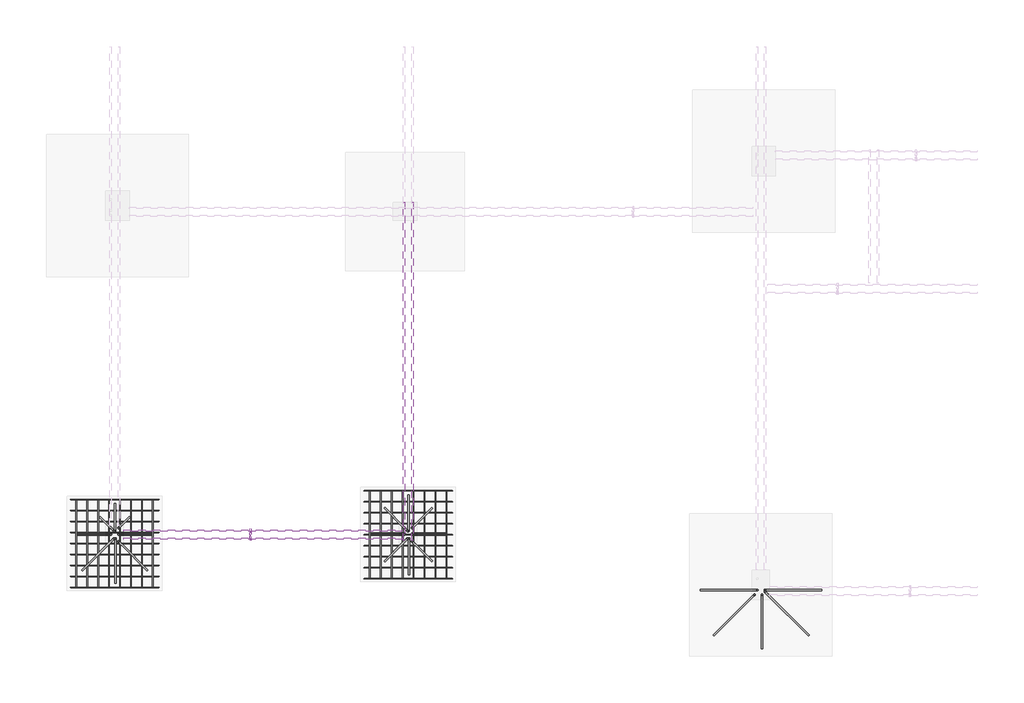
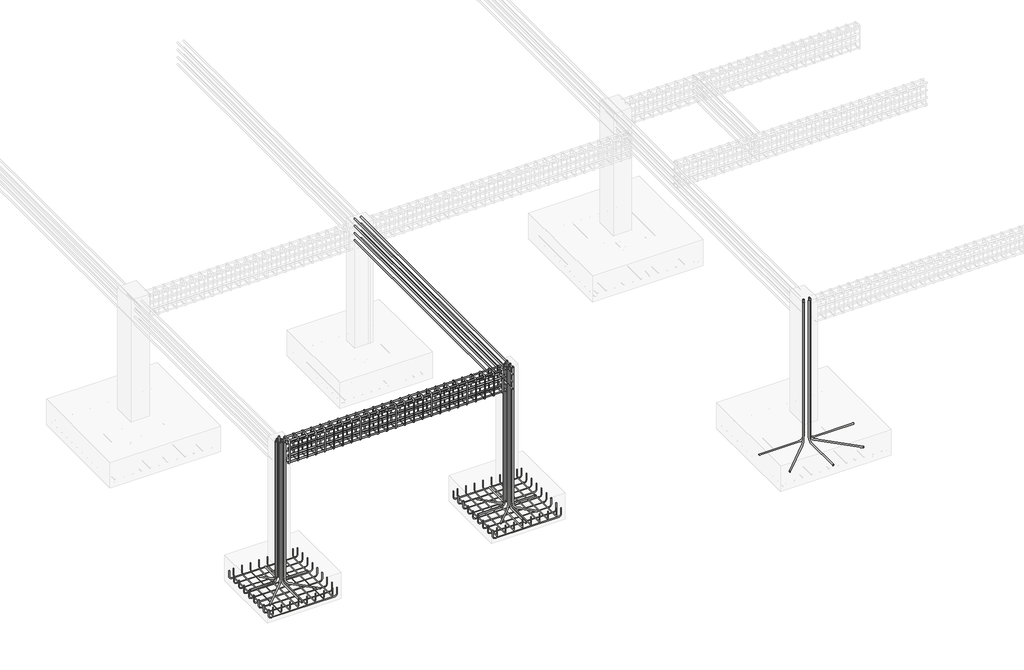
# One storey, part 2 of 10: 34 reinforcing bars.
"""IFC4 building model written with IfcOpenShell, lengths in millimetres."""

from ifc_helpers import new_model, si_unit, point, frame, origin, place, context, project, spatial, polyline, circle_curve, trimmed, segment, composite_curve, source, transform, mapped, element, save
from ifc_brep_helpers import swept_disk

model = new_model("IFC4")

# Units and contexts
model_context = context("Model", 3, world=origin())
ifc_project = project(units=[si_unit("LENGTHUNIT", "METRE", prefix="MILLI")], contexts=[model_context])

# Site, building, storey
site = spatial("IfcSite", under=ifc_project)
building = spatial("IfcBuilding", under=site)
storey = spatial("IfcBuildingStorey", under=building, Elevation=-2133.6)

# Reinforcing bars
placement = place(None, origin())
reinforcing_bar_shape = source(origin(), model_context, "Body", "SolidModel", [
    swept_disk(composite_curve([segment(polyline([(-4370.4164362, -2867.2780823, -2393.6), (-4370.4164362, -2867.2780823, -2504.1)]), True, "CONTINUOUS"), segment(trimmed(circle_curve(frame((-4405.1664362, -2867.2780823, -2504.1), z_axis=(0.0, 1.0, 0.0), x_axis=(34.75, 0.0, 0.0)), 34.75), [point((-4370.4164362, -2867.2780823, -2504.1))], [point((-4405.1664362, -2867.2780823, -2538.85))], True, "CARTESIAN"), True, "CONTINUOUS"), segment(polyline([(-4405.1664362, -2867.2780823, -2538.85), (-5465.3664362, -2867.2780823, -2538.85)]), True, "CONTINUOUS"), segment(trimmed(circle_curve(frame((-5465.3664362, -2867.2780823, -2504.1), z_axis=(0.0, 1.0, 0.0), x_axis=(0.0, 0.0, -34.75)), 34.75), [point((-5465.3664362, -2867.2780823, -2538.85))], [point((-5500.1164362, -2867.2780823, -2504.1))], True, "CARTESIAN"), True, "CONTINUOUS"), segment(polyline([(-5500.1164362, -2867.2780823, -2504.1), (-5500.1164362, -2867.2780823, -2393.6)]), True, "CONTINUOUS")], self_intersect=False), 4.75),
])
element("IfcReinforcingBar", 1, at=placement, inside=storey, context=model_context, shape_type="MappedRepresentation", body=[
    mapped(reinforcing_bar_shape, transform((0.0, 0.0, 0.0), x_axis=(1.0, 0.0, 0.0), y_axis=(0.0, 1.0, 0.0), z_axis=(0.0, 0.0, 1.0))),
    mapped(reinforcing_bar_shape, transform((0.0, -141.2125, 0.0), x_axis=(1.0, 0.0, 0.0), y_axis=(0.0, 1.0, 0.0), z_axis=(0.0, 0.0, 1.0))),
    mapped(reinforcing_bar_shape, transform((0.0, -282.425, 0.0), x_axis=(1.0, 0.0, 0.0), y_axis=(0.0, 1.0, 0.0), z_axis=(0.0, 0.0, 1.0))),
    mapped(reinforcing_bar_shape, transform((0.0, -423.6375, 0.0), x_axis=(1.0, 0.0, 0.0), y_axis=(0.0, 1.0, 0.0), z_axis=(0.0, 0.0, 1.0))),
    mapped(reinforcing_bar_shape, transform((0.0, -564.85, 0.0), x_axis=(1.0, 0.0, 0.0), y_axis=(0.0, 1.0, 0.0), z_axis=(0.0, 0.0, 1.0))),
    mapped(reinforcing_bar_shape, transform((0.0, -706.0625, 0.0), x_axis=(1.0, 0.0, 0.0), y_axis=(0.0, 1.0, 0.0), z_axis=(0.0, 0.0, 1.0))),
    mapped(reinforcing_bar_shape, transform((0.0, -847.275, 0.0), x_axis=(1.0, 0.0, 0.0), y_axis=(0.0, 1.0, 0.0), z_axis=(0.0, 0.0, 1.0))),
    mapped(reinforcing_bar_shape, transform((0.0, -988.4875, 0.0), x_axis=(1.0, 0.0, 0.0), y_axis=(0.0, 1.0, 0.0), z_axis=(0.0, 0.0, 1.0))),
    mapped(reinforcing_bar_shape, transform((0.0, -1129.7, 0.0), x_axis=(1.0, 0.0, 0.0), y_axis=(0.0, 1.0, 0.0), z_axis=(0.0, 0.0, 1.0))),
])
reinforcing_bar_2_shape = source(origin(), model_context, "Body", "SolidModel", [
    swept_disk(composite_curve([segment(polyline([(-4445.3743867, -3996.9780823, -2379.223371), (-4445.3743867, -3996.9780823, -2489.723371)]), True, "CONTINUOUS"), segment(trimmed(circle_curve(frame((-4445.3743867, -3962.2280823, -2489.723371), z_axis=(1.0, 0.0, 0.0), x_axis=(0.0, -34.75, 0.0)), 34.75), [point((-4445.3743867, -3996.9780823, -2489.723371))], [point((-4445.3743867, -3962.2280823, -2524.473371))], True, "CARTESIAN"), True, "CONTINUOUS"), segment(polyline([(-4445.3743867, -3962.2280823, -2524.473371), (-4445.3743867, -2902.0280823, -2524.473371)]), True, "CONTINUOUS"), segment(trimmed(circle_curve(frame((-4445.3743867, -2902.0280823, -2489.723371), z_axis=(1.0, 0.0, 0.0), x_axis=(0.0, 0.0, -34.75)), 34.75), [point((-4445.3743867, -2902.0280823, -2524.473371))], [point((-4445.3743867, -2867.2780823, -2489.723371))], True, "CARTESIAN"), True, "CONTINUOUS"), segment(polyline([(-4445.3743867, -2867.2780823, -2489.723371), (-4445.3743867, -2867.2780823, -2379.223371)]), True, "CONTINUOUS")], self_intersect=False), 4.75),
])
element("IfcReinforcingBar", 2, at=placement, inside=storey, context=model_context, shape_type="MappedRepresentation", body=[
    mapped(reinforcing_bar_2_shape, transform((0.0, 0.0, 0.0), x_axis=(1.0, 0.0, 0.0), y_axis=(0.0, 1.0, 0.0), z_axis=(0.0, 0.0, 1.0))),
    mapped(reinforcing_bar_2_shape, transform((-140.5079612, 0.0, 0.0), x_axis=(1.0, 0.0, 0.0), y_axis=(0.0, 1.0, 0.0), z_axis=(0.0, 0.0, 1.0))),
    mapped(reinforcing_bar_2_shape, transform((-281.0159224, 0.0, 0.0), x_axis=(1.0, 0.0, 0.0), y_axis=(0.0, 1.0, 0.0), z_axis=(0.0, 0.0, 1.0))),
    mapped(reinforcing_bar_2_shape, transform((-421.5238836, 0.0, 0.0), x_axis=(1.0, 0.0, 0.0), y_axis=(0.0, 1.0, 0.0), z_axis=(0.0, 0.0, 1.0))),
    mapped(reinforcing_bar_2_shape, transform((-562.0318448, 0.0, 0.0), x_axis=(1.0, 0.0, 0.0), y_axis=(0.0, 1.0, 0.0), z_axis=(0.0, 0.0, 1.0))),
    mapped(reinforcing_bar_2_shape, transform((-702.539806, 0.0, 0.0), x_axis=(1.0, 0.0, 0.0), y_axis=(0.0, 1.0, 0.0), z_axis=(0.0, 0.0, 1.0))),
    mapped(reinforcing_bar_2_shape, transform((-843.0477672, 0.0, 0.0), x_axis=(1.0, 0.0, 0.0), y_axis=(0.0, 1.0, 0.0), z_axis=(0.0, 0.0, 1.0))),
    mapped(reinforcing_bar_2_shape, transform((-983.5557284, 0.0, 0.0), x_axis=(1.0, 0.0, 0.0), y_axis=(0.0, 1.0, 0.0), z_axis=(0.0, 0.0, 1.0))),
])
reinforcing_bar_3_shape = source(origin(), model_context, "Body", "SolidModel", [
    swept_disk(composite_curve([segment(polyline([(-598.5164362, -2752.9780823, -2393.6), (-598.5164362, -2752.9780823, -2504.1)]), True, "CONTINUOUS"), segment(trimmed(circle_curve(frame((-633.2664362, -2752.9780823, -2504.1), z_axis=(0.0, 1.0, 0.0), x_axis=(34.75, 0.0, 0.0)), 34.75), [point((-598.5164362, -2752.9780823, -2504.1))], [point((-633.2664362, -2752.9780823, -2538.85))], True, "CARTESIAN"), True, "CONTINUOUS"), segment(polyline([(-633.2664362, -2752.9780823, -2538.85), (-1693.4664362, -2752.9780823, -2538.85)]), True, "CONTINUOUS"), segment(trimmed(circle_curve(frame((-1693.4664362, -2752.9780823, -2504.1), z_axis=(0.0, 1.0, 0.0), x_axis=(0.0, 0.0, -34.75)), 34.75), [point((-1693.4664362, -2752.9780823, -2538.85))], [point((-1728.2164362, -2752.9780823, -2504.1))], True, "CARTESIAN"), True, "CONTINUOUS"), segment(polyline([(-1728.2164362, -2752.9780823, -2504.1), (-1728.2164362, -2752.9780823, -2393.6)]), True, "CONTINUOUS")], self_intersect=False), 4.75),
])
element("IfcReinforcingBar", 3, at=placement, inside=storey, context=model_context, shape_type="MappedRepresentation", body=[
    mapped(reinforcing_bar_3_shape, transform((0.0, 0.0, 0.0), x_axis=(1.0, 0.0, 0.0), y_axis=(0.0, 1.0, 0.0), z_axis=(0.0, 0.0, 1.0))),
    mapped(reinforcing_bar_3_shape, transform((0.0, -141.2125, 0.0), x_axis=(1.0, 0.0, 0.0), y_axis=(0.0, 1.0, 0.0), z_axis=(0.0, 0.0, 1.0))),
    mapped(reinforcing_bar_3_shape, transform((0.0, -282.425, 0.0), x_axis=(1.0, 0.0, 0.0), y_axis=(0.0, 1.0, 0.0), z_axis=(0.0, 0.0, 1.0))),
    mapped(reinforcing_bar_3_shape, transform((0.0, -423.6375, 0.0), x_axis=(1.0, 0.0, 0.0), y_axis=(0.0, 1.0, 0.0), z_axis=(0.0, 0.0, 1.0))),
    mapped(reinforcing_bar_3_shape, transform((0.0, -564.85, 0.0), x_axis=(1.0, 0.0, 0.0), y_axis=(0.0, 1.0, 0.0), z_axis=(0.0, 0.0, 1.0))),
    mapped(reinforcing_bar_3_shape, transform((0.0, -706.0625, 0.0), x_axis=(1.0, 0.0, 0.0), y_axis=(0.0, 1.0, 0.0), z_axis=(0.0, 0.0, 1.0))),
    mapped(reinforcing_bar_3_shape, transform((0.0, -847.275, 0.0), x_axis=(1.0, 0.0, 0.0), y_axis=(0.0, 1.0, 0.0), z_axis=(0.0, 0.0, 1.0))),
    mapped(reinforcing_bar_3_shape, transform((0.0, -988.4875, 0.0), x_axis=(1.0, 0.0, 0.0), y_axis=(0.0, 1.0, 0.0), z_axis=(0.0, 0.0, 1.0))),
    mapped(reinforcing_bar_3_shape, transform((0.0, -1129.7, 0.0), x_axis=(1.0, 0.0, 0.0), y_axis=(0.0, 1.0, 0.0), z_axis=(0.0, 0.0, 1.0))),
])
reinforcing_bar_4_shape = source(origin(), model_context, "Body", "SolidModel", [
    swept_disk(composite_curve([segment(polyline([(-673.4743867, -3882.6780823, -2379.223371), (-673.4743867, -3882.6780823, -2489.723371)]), True, "CONTINUOUS"), segment(trimmed(circle_curve(frame((-673.4743867, -3847.9280823, -2489.723371), z_axis=(1.0, 0.0, 0.0), x_axis=(0.0, -34.75, 0.0)), 34.75), [point((-673.4743867, -3882.6780823, -2489.723371))], [point((-673.4743867, -3847.9280823, -2524.473371))], True, "CARTESIAN"), True, "CONTINUOUS"), segment(polyline([(-673.4743867, -3847.9280823, -2524.473371), (-673.4743867, -2787.7280823, -2524.473371)]), True, "CONTINUOUS"), segment(trimmed(circle_curve(frame((-673.4743867, -2787.7280823, -2489.723371), z_axis=(1.0, 0.0, 0.0), x_axis=(0.0, 0.0, -34.75)), 34.75), [point((-673.4743867, -2787.7280823, -2524.473371))], [point((-673.4743867, -2752.9780823, -2489.723371))], True, "CARTESIAN"), True, "CONTINUOUS"), segment(polyline([(-673.4743867, -2752.9780823, -2489.723371), (-673.4743867, -2752.9780823, -2379.223371)]), True, "CONTINUOUS")], self_intersect=False), 4.75),
])
element("IfcReinforcingBar", 4, at=placement, inside=storey, context=model_context, shape_type="MappedRepresentation", body=[
    mapped(reinforcing_bar_4_shape, transform((0.0, 0.0, 0.0), x_axis=(1.0, 0.0, 0.0), y_axis=(0.0, 1.0, 0.0), z_axis=(0.0, 0.0, 1.0))),
    mapped(reinforcing_bar_4_shape, transform((-140.5079612, 0.0, 0.0), x_axis=(1.0, 0.0, 0.0), y_axis=(0.0, 1.0, 0.0), z_axis=(0.0, 0.0, 1.0))),
    mapped(reinforcing_bar_4_shape, transform((-281.0159224, 0.0, 0.0), x_axis=(1.0, 0.0, 0.0), y_axis=(0.0, 1.0, 0.0), z_axis=(0.0, 0.0, 1.0))),
    mapped(reinforcing_bar_4_shape, transform((-421.5238836, 0.0, 0.0), x_axis=(1.0, 0.0, 0.0), y_axis=(0.0, 1.0, 0.0), z_axis=(0.0, 0.0, 1.0))),
    mapped(reinforcing_bar_4_shape, transform((-562.0318448, 0.0, 0.0), x_axis=(1.0, 0.0, 0.0), y_axis=(0.0, 1.0, 0.0), z_axis=(0.0, 0.0, 1.0))),
    mapped(reinforcing_bar_4_shape, transform((-702.539806, 0.0, 0.0), x_axis=(1.0, 0.0, 0.0), y_axis=(0.0, 1.0, 0.0), z_axis=(0.0, 0.0, 1.0))),
    mapped(reinforcing_bar_4_shape, transform((-843.0477672, 0.0, 0.0), x_axis=(1.0, 0.0, 0.0), y_axis=(0.0, 1.0, 0.0), z_axis=(0.0, 0.0, 1.0))),
    mapped(reinforcing_bar_4_shape, transform((-983.5557284, 0.0, 0.0), x_axis=(1.0, 0.0, 0.0), y_axis=(0.0, 1.0, 0.0), z_axis=(0.0, 0.0, 1.0))),
])
element("IfcReinforcingBar", 5, at=placement, inside=storey, context=model_context, shape_type="SolidModel", body=[
    swept_disk(composite_curve([segment(polyline([(3285.2335638, -4089.8114607, -40.0), (3285.2335638, -4089.8114607, -2426.55)]), True, "CONTINUOUS"), segment(trimmed(circle_curve(frame((3237.8220542, -4137.2229704, -2426.55), z_axis=(-0.707106781186552, 0.7071067811865431, 0.0), x_axis=(47.411509600000045, 47.4115096999999, 0.0)), 67.05), [point((3285.2335638, -4089.8114607, -2426.55))], [point((3237.8220542, -4137.2229704, -2493.6))], True, "CARTESIAN"), True, "CONTINUOUS"), segment(polyline([(3237.8220542, -4137.2229704, -2493.6), (2760.8116308, -4614.2333938, -2493.6)]), True, "CONTINUOUS")], self_intersect=False), 9.55),
])
element("IfcReinforcingBar", 6, at=placement, inside=storey, context=model_context, shape_type="SolidModel", body=[
    swept_disk(composite_curve([segment(polyline([(3418.8335638, -4051.7114607, -40.0), (3418.8335638, -4051.7114607, -2426.55)]), True, "CONTINUOUS"), segment(trimmed(circle_curve(frame((3466.2450735, -4099.1229704, -2426.55), z_axis=(-0.707106781186552, -0.7071067811865431, 0.0), x_axis=(-47.41150970000035, 47.4115096999999, 0.0)), 67.05), [point((3418.8335638, -4051.7114607, -2426.55))], [point((3466.2450735, -4099.1229704, -2493.6))], True, "CARTESIAN"), True, "CONTINUOUS"), segment(polyline([(3466.2450735, -4099.1229704, -2493.6), (3981.3554969, -4614.2333938, -2493.6)]), True, "CONTINUOUS")], self_intersect=False), 9.55),
])
element("IfcReinforcingBar", 7, at=placement, inside=storey, context=model_context, shape_type="SolidModel", body=[
    swept_disk(composite_curve([segment(polyline([(3382.2194855, -4089.8114607, -40.0), (3382.2194855, -4089.8114607, -2426.55)]), True, "CONTINUOUS"), segment(trimmed(circle_curve(frame((3382.2194855, -4156.8614607, -2426.55), z_axis=(-1.0, 0.0, 0.0), x_axis=(0.0, 67.04999999999973, 0.0)), 67.05), [point((3382.2194855, -4089.8114607, -2426.55))], [point((3382.2194855, -4156.8614607, -2493.6))], True, "CARTESIAN"), True, "CONTINUOUS"), segment(polyline([(3382.2194855, -4156.8614607, -2493.6), (3382.2194855, -4784.1114607, -2493.6)]), True, "CONTINUOUS")], self_intersect=False), 9.55),
])
element("IfcReinforcingBar", 8, at=placement, inside=storey, context=model_context, shape_type="SolidModel", body=[
    swept_disk(composite_curve([segment(polyline([(3323.3335638, -4029.5829002, -40.0), (3323.3335638, -4029.5829002, -2426.55)]), True, "CONTINUOUS"), segment(trimmed(circle_curve(frame((3256.2835638, -4029.5829002, -2426.55), z_axis=(0.0, 1.0, 0.0), x_axis=(67.04999999999973, 0.0, 0.0)), 67.05), [point((3323.3335638, -4029.5829002, -2426.55))], [point((3256.2835638, -4029.5829002, -2493.6))], True, "CARTESIAN"), True, "CONTINUOUS"), segment(polyline([(3256.2835638, -4029.5829002, -2493.6), (2590.9335638, -4029.5829002, -2493.6)]), True, "CONTINUOUS")], self_intersect=False), 9.55),
])
element("IfcReinforcingBar", 9, at=placement, inside=storey, context=model_context, shape_type="SolidModel", body=[
    swept_disk(composite_curve([segment(polyline([(3418.8335638, -4029.5829002, -40.0), (3418.8335638, -4029.5829002, -2426.55)]), True, "CONTINUOUS"), segment(trimmed(circle_curve(frame((3485.8835638, -4029.5829002, -2426.55), z_axis=(0.0, -1.0, 0.0), x_axis=(-67.05000000000018, 0.0, 0.0)), 67.05), [point((3418.8335638, -4029.5829002, -2426.55))], [point((3485.8835638, -4029.5829002, -2493.6))], True, "CARTESIAN"), True, "CONTINUOUS"), segment(polyline([(3485.8835638, -4029.5829002, -2493.6), (4151.2335638, -4029.5829002, -2493.6)]), True, "CONTINUOUS")], self_intersect=False), 9.55),
])
element("IfcReinforcingBar", 10, at=placement, inside=storey, context=model_context, shape_type="SolidModel", body=[
    swept_disk(composite_curve([segment(polyline([(-1172.4664362, -3269.7447039, -40.0), (-1172.4664362, -3269.7447039, -2426.55)]), True, "CONTINUOUS"), segment(trimmed(circle_curve(frame((-1219.8779458, -3222.3331942, -2426.55), z_axis=(0.7071067811865519, 0.7071067811865431, 0.0), x_axis=(47.41150959999982, -47.4115096999999, 0.0)), 67.05), [point((-1172.4664362, -3269.7447039, -2426.55))], [point((-1219.8779458, -3222.3331942, -2493.6))], True, "CARTESIAN"), True, "CONTINUOUS"), segment(polyline([(-1219.8779458, -3222.3331942, -2493.6), (-1468.2883692, -2973.9227708, -2493.6)]), True, "CONTINUOUS")], self_intersect=False), 9.55),
])
element("IfcReinforcingBar", 11, at=placement, inside=storey, context=model_context, shape_type="SolidModel", body=[
    swept_disk(composite_curve([segment(polyline([(-1115.0664362, -3231.6447039, -40.0), (-1115.0664362, -3231.6447039, -2426.55)]), True, "CONTINUOUS"), segment(trimmed(circle_curve(frame((-1067.6549265, -3184.2331942, -2426.55), z_axis=(0.7071067811865519, -0.7071067811865431, 0.0), x_axis=(-47.4115096999999, -47.4115096999999, 0.0)), 67.05), [point((-1115.0664362, -3231.6447039, -2426.55))], [point((-1067.6549265, -3184.2331942, -2493.6))], True, "CARTESIAN"), True, "CONTINUOUS"), segment(polyline([(-1067.6549265, -3184.2331942, -2493.6), (-857.3445031, -2973.9227708, -2493.6)]), True, "CONTINUOUS")], self_intersect=False), 9.55),
])
element("IfcReinforcingBar", 12, at=placement, inside=storey, context=model_context, shape_type="SolidModel", body=[
    swept_disk(composite_curve([segment(polyline([(-1172.4664362, -3365.9114607, -40.0), (-1172.4664362, -3365.9114607, -2426.55)]), True, "CONTINUOUS"), segment(trimmed(circle_curve(frame((-1219.8779458, -3413.3229704, -2426.55), z_axis=(-0.7071067811865519, 0.7071067811865431, 0.0), x_axis=(47.41150959999982, 47.4115096999999, 0.0)), 67.05), [point((-1172.4664362, -3365.9114607, -2426.55))], [point((-1219.8779458, -3413.3229704, -2493.6))], True, "CARTESIAN"), True, "CONTINUOUS"), segment(polyline([(-1219.8779458, -3413.3229704, -2493.6), (-1468.2883692, -3661.7333938, -2493.6)]), True, "CONTINUOUS")], self_intersect=False), 9.55),
])
element("IfcReinforcingBar", 13, at=placement, inside=storey, context=model_context, shape_type="SolidModel", body=[
    swept_disk(composite_curve([segment(polyline([(-1115.0664362, -3404.0114607, -40.0), (-1115.0664362, -3404.0114607, -2426.55)]), True, "CONTINUOUS"), segment(trimmed(circle_curve(frame((-1067.6549265, -3451.4229704, -2426.55), z_axis=(-0.7071067811865519, -0.7071067811865431, 0.0), x_axis=(-47.4115096999999, 47.4115096999999, 0.0)), 67.05), [point((-1115.0664362, -3404.0114607, -2426.55))], [point((-1067.6549265, -3451.4229704, -2493.6))], True, "CARTESIAN"), True, "CONTINUOUS"), segment(polyline([(-1067.6549265, -3451.4229704, -2493.6), (-857.3445031, -3661.7333938, -2493.6)]), True, "CONTINUOUS")], self_intersect=False), 9.55),
])
element("IfcReinforcingBar", 14, at=placement, inside=storey, context=model_context, shape_type="SolidModel", body=[
    swept_disk(composite_curve([segment(polyline([(-1161.6805145, -3269.7447039, -40.0), (-1161.6805145, -3269.7447039, -2426.55)]), True, "CONTINUOUS"), segment(trimmed(circle_curve(frame((-1161.6805145, -3202.6947039, -2426.55), z_axis=(1.0, 0.0, 0.0), x_axis=(0.0, -67.04999999999973, 0.0)), 67.05), [point((-1161.6805145, -3269.7447039, -2426.55))], [point((-1161.6805145, -3202.6947039, -2493.6))], True, "CARTESIAN"), True, "CONTINUOUS"), segment(polyline([(-1161.6805145, -3202.6947039, -2493.6), (-1161.6805145, -2804.0447039, -2493.6)]), True, "CONTINUOUS")], self_intersect=False), 9.55),
])
element("IfcReinforcingBar", 15, at=placement, inside=storey, context=model_context, shape_type="SolidModel", body=[
    swept_disk(composite_curve([segment(polyline([(-1151.6805145, -3365.9114607, -40.0), (-1151.6805145, -3365.9114607, -2426.55)]), True, "CONTINUOUS"), segment(trimmed(circle_curve(frame((-1151.6805145, -3432.9614607, -2426.55), z_axis=(-1.0, 0.0, 0.0), x_axis=(0.0, 67.04999999999973, 0.0)), 67.05), [point((-1151.6805145, -3365.9114607, -2426.55))], [point((-1151.6805145, -3432.9614607, -2493.6))], True, "CARTESIAN"), True, "CONTINUOUS"), segment(polyline([(-1151.6805145, -3432.9614607, -2493.6), (-1151.6805145, -3831.6114607, -2493.6)]), True, "CONTINUOUS")], self_intersect=False), 9.55),
])
element("IfcReinforcingBar", 16, at=placement, inside=storey, context=model_context, shape_type="SolidModel", body=[
    swept_disk(composite_curve([segment(polyline([(-1210.5664362, -3314.7447039, -40.0), (-1210.5664362, -3314.7447039, -2426.55)]), True, "CONTINUOUS"), segment(trimmed(circle_curve(frame((-1277.6164362, -3314.7447039, -2426.55), z_axis=(0.0, 1.0, 0.0), x_axis=(67.04999999999995, 0.0, 0.0)), 67.05), [point((-1210.5664362, -3314.7447039, -2426.55))], [point((-1277.6164362, -3314.7447039, -2493.6))], True, "CARTESIAN"), True, "CONTINUOUS"), segment(polyline([(-1277.6164362, -3314.7447039, -2493.6), (-1638.1664362, -3314.7447039, -2493.6)]), True, "CONTINUOUS")], self_intersect=False), 9.55),
])
element("IfcReinforcingBar", 17, at=placement, inside=storey, context=model_context, shape_type="SolidModel", body=[
    swept_disk(composite_curve([segment(polyline([(-1210.5664362, -3305.6829002, -40.0), (-1210.5664362, -3305.6829002, -2426.55)]), True, "CONTINUOUS"), segment(trimmed(circle_curve(frame((-1277.6164362, -3305.6829002, -2426.55), z_axis=(0.0, 1.0, 0.0), x_axis=(67.04999999999995, 0.0, 0.0)), 67.05), [point((-1210.5664362, -3305.6829002, -2426.55))], [point((-1277.6164362, -3305.6829002, -2493.6))], True, "CARTESIAN"), True, "CONTINUOUS"), segment(polyline([(-1277.6164362, -3305.6829002, -2493.6), (-1638.1664362, -3305.6829002, -2493.6)]), True, "CONTINUOUS")], self_intersect=False), 9.55),
])
element("IfcReinforcingBar", 18, at=placement, inside=storey, context=model_context, shape_type="SolidModel", body=[
    swept_disk(composite_curve([segment(polyline([(-1115.0664362, -3314.7447039, -40.0), (-1115.0664362, -3314.7447039, -2426.55)]), True, "CONTINUOUS"), segment(trimmed(circle_curve(frame((-1048.0164362, -3314.7447039, -2426.55), z_axis=(0.0, -1.0, 0.0), x_axis=(-67.04999999999995, 0.0, 0.0)), 67.05), [point((-1115.0664362, -3314.7447039, -2426.55))], [point((-1048.0164362, -3314.7447039, -2493.6))], True, "CARTESIAN"), True, "CONTINUOUS"), segment(polyline([(-1048.0164362, -3314.7447039, -2493.6), (-687.4664362, -3314.7447039, -2493.6)]), True, "CONTINUOUS")], self_intersect=False), 9.55),
])
element("IfcReinforcingBar", 19, at=placement, inside=storey, context=model_context, shape_type="SolidModel", body=[
    swept_disk(composite_curve([segment(polyline([(-1115.0664362, -3305.6829002, -40.0), (-1115.0664362, -3305.6829002, -2426.55)]), True, "CONTINUOUS"), segment(trimmed(circle_curve(frame((-1048.0164362, -3305.6829002, -2426.55), z_axis=(0.0, -1.0, 0.0), x_axis=(-67.04999999999995, 0.0, 0.0)), 67.05), [point((-1115.0664362, -3305.6829002, -2426.55))], [point((-1048.0164362, -3305.6829002, -2493.6))], True, "CARTESIAN"), True, "CONTINUOUS"), segment(polyline([(-1048.0164362, -3305.6829002, -2493.6), (-687.4664362, -3305.6829002, -2493.6)]), True, "CONTINUOUS")], self_intersect=False), 9.55),
])
element("IfcReinforcingBar", 20, at=placement, inside=storey, context=model_context, shape_type="SolidModel", body=[
    swept_disk(composite_curve([segment(polyline([(-4944.3664362, -3269.7447039, -40.0), (-4944.3664362, -3269.7447039, -2426.55)]), True, "CONTINUOUS"), segment(trimmed(circle_curve(frame((-4991.7779458, -3222.3331942, -2426.55), z_axis=(0.7071067811865519, 0.7071067811865431, 0.0), x_axis=(47.4115096000005, -47.4115096999999, 0.0)), 67.05), [point((-4944.3664362, -3269.7447039, -2426.55))], [point((-4991.7779458, -3222.3331942, -2493.6))], True, "CARTESIAN"), True, "CONTINUOUS"), segment(polyline([(-4991.7779458, -3222.3331942, -2493.6), (-5125.8883692, -3088.2227708, -2493.6)]), True, "CONTINUOUS")], self_intersect=False), 9.55),
])
element("IfcReinforcingBar", 21, at=placement, inside=storey, context=model_context, shape_type="SolidModel", body=[
    swept_disk(composite_curve([segment(polyline([(-4886.9664362, -3231.6447039, -40.0), (-4886.9664362, -3231.6447039, -2426.55)]), True, "CONTINUOUS"), segment(trimmed(circle_curve(frame((-4839.5549265, -3184.2331942, -2426.55), z_axis=(0.7071067811865519, -0.7071067811865431, 0.0), x_axis=(-47.41150970000035, -47.4115096999999, 0.0)), 67.05), [point((-4886.9664362, -3231.6447039, -2426.55))], [point((-4839.5549265, -3184.2331942, -2493.6))], True, "CARTESIAN"), True, "CONTINUOUS"), segment(polyline([(-4839.5549265, -3184.2331942, -2493.6), (-4743.5445031, -3088.2227708, -2493.6)]), True, "CONTINUOUS")], self_intersect=False), 9.55),
])
element("IfcReinforcingBar", 22, at=placement, inside=storey, context=model_context, shape_type="SolidModel", body=[
    swept_disk(composite_curve([segment(polyline([(-4944.3664362, -3365.9114607, -40.0), (-4944.3664362, -3365.9114607, -2426.55)]), True, "CONTINUOUS"), segment(trimmed(circle_curve(frame((-4991.7779458, -3413.3229704, -2426.55), z_axis=(-0.7071067811865519, 0.7071067811865431, 0.0), x_axis=(47.4115096000005, 47.4115096999999, 0.0)), 67.05), [point((-4944.3664362, -3365.9114607, -2426.55))], [point((-4991.7779458, -3413.3229704, -2493.6))], True, "CARTESIAN"), True, "CONTINUOUS"), segment(polyline([(-4991.7779458, -3413.3229704, -2493.6), (-5354.4883692, -3776.0333938, -2493.6)]), True, "CONTINUOUS")], self_intersect=False), 9.55),
])
element("IfcReinforcingBar", 23, at=placement, inside=storey, context=model_context, shape_type="SolidModel", body=[
    swept_disk(composite_curve([segment(polyline([(-4886.9664362, -3404.0114607, -40.0), (-4886.9664362, -3404.0114607, -2426.55)]), True, "CONTINUOUS"), segment(trimmed(circle_curve(frame((-4839.5549265, -3451.4229704, -2426.55), z_axis=(-0.7071067811865519, -0.7071067811865431, 0.0), x_axis=(-47.41150970000035, 47.4115096999999, 0.0)), 67.05), [point((-4886.9664362, -3404.0114607, -2426.55))], [point((-4839.5549265, -3451.4229704, -2493.6))], True, "CARTESIAN"), True, "CONTINUOUS"), segment(polyline([(-4839.5549265, -3451.4229704, -2493.6), (-4514.9445031, -3776.0333938, -2493.6)]), True, "CONTINUOUS")], self_intersect=False), 9.55),
])
element("IfcReinforcingBar", 24, at=placement, inside=storey, context=model_context, shape_type="SolidModel", body=[
    swept_disk(composite_curve([segment(polyline([(-4933.5805145, -3269.7447039, -40.0), (-4933.5805145, -3269.7447039, -2426.55)]), True, "CONTINUOUS"), segment(trimmed(circle_curve(frame((-4933.5805145, -3202.6947039, -2426.55), z_axis=(1.0, 0.0, 0.0), x_axis=(0.0, -67.04999999999973, 0.0)), 67.05), [point((-4933.5805145, -3269.7447039, -2426.55))], [point((-4933.5805145, -3202.6947039, -2493.6))], True, "CARTESIAN"), True, "CONTINUOUS"), segment(polyline([(-4933.5805145, -3202.6947039, -2493.6), (-4933.5805145, -2918.3447039, -2493.6)]), True, "CONTINUOUS")], self_intersect=False), 9.55),
])
element("IfcReinforcingBar", 25, at=placement, inside=storey, context=model_context, shape_type="SolidModel", body=[
    swept_disk(composite_curve([segment(polyline([(-4923.5805145, -3365.9114607, -40.0), (-4923.5805145, -3365.9114607, -2426.55)]), True, "CONTINUOUS"), segment(trimmed(circle_curve(frame((-4923.5805145, -3432.9614607, -2426.55), z_axis=(-1.0, 0.0, 0.0), x_axis=(0.0, 67.04999999999973, 0.0)), 67.05), [point((-4923.5805145, -3365.9114607, -2426.55))], [point((-4923.5805145, -3432.9614607, -2493.6))], True, "CARTESIAN"), True, "CONTINUOUS"), segment(polyline([(-4923.5805145, -3432.9614607, -2493.6), (-4923.5805145, -3945.9114607, -2493.6)]), True, "CONTINUOUS")], self_intersect=False), 9.55),
])
element("IfcReinforcingBar", 26, at=placement, inside=storey, context=model_context, shape_type="SolidModel", body=[
    swept_disk(composite_curve([segment(polyline([(-4982.4664362, -3314.7447039, -40.0), (-4982.4664362, -3314.7447039, -2426.55)]), True, "CONTINUOUS"), segment(trimmed(circle_curve(frame((-5049.5164362, -3314.7447039, -2426.55), z_axis=(0.0, 1.0, 0.0), x_axis=(67.04999999999927, 0.0, 0.0)), 67.05), [point((-4982.4664362, -3314.7447039, -2426.55))], [point((-5049.5164362, -3314.7447039, -2493.6))], True, "CARTESIAN"), True, "CONTINUOUS"), segment(polyline([(-5049.5164362, -3314.7447039, -2493.6), (-5410.0664362, -3314.7447039, -2493.6)]), True, "CONTINUOUS")], self_intersect=False), 9.55),
])
element("IfcReinforcingBar", 27, at=placement, inside=storey, context=model_context, shape_type="SolidModel", body=[
    swept_disk(composite_curve([segment(polyline([(-4982.4664362, -3305.6829002, -40.0), (-4982.4664362, -3305.6829002, -2426.55)]), True, "CONTINUOUS"), segment(trimmed(circle_curve(frame((-5049.5164362, -3305.6829002, -2426.55), z_axis=(0.0, 1.0, 0.0), x_axis=(67.04999999999927, 0.0, 0.0)), 67.05), [point((-4982.4664362, -3305.6829002, -2426.55))], [point((-5049.5164362, -3305.6829002, -2493.6))], True, "CARTESIAN"), True, "CONTINUOUS"), segment(polyline([(-5049.5164362, -3305.6829002, -2493.6), (-5410.0664362, -3305.6829002, -2493.6)]), True, "CONTINUOUS")], self_intersect=False), 9.55),
])
element("IfcReinforcingBar", 28, at=placement, inside=storey, context=model_context, shape_type="SolidModel", body=[
    swept_disk(composite_curve([segment(polyline([(-4886.9664362, -3314.7447039, -40.0), (-4886.9664362, -3314.7447039, -2426.55)]), True, "CONTINUOUS"), segment(trimmed(circle_curve(frame((-4819.9164362, -3314.7447039, -2426.55), z_axis=(0.0, -1.0, 0.0), x_axis=(-67.05000000000018, 0.0, 0.0)), 67.05), [point((-4886.9664362, -3314.7447039, -2426.55))], [point((-4819.9164362, -3314.7447039, -2493.6))], True, "CARTESIAN"), True, "CONTINUOUS"), segment(polyline([(-4819.9164362, -3314.7447039, -2493.6), (-4459.3664362, -3314.7447039, -2493.6)]), True, "CONTINUOUS")], self_intersect=False), 9.55),
])
element("IfcReinforcingBar", 29, at=placement, inside=storey, context=model_context, shape_type="SolidModel", body=[
    swept_disk(composite_curve([segment(polyline([(-4886.9664362, -3305.6829002, -40.0), (-4886.9664362, -3305.6829002, -2426.55)]), True, "CONTINUOUS"), segment(trimmed(circle_curve(frame((-4819.9164362, -3305.6829002, -2426.55), z_axis=(0.0, -1.0, 0.0), x_axis=(-67.05000000000018, 0.0, 0.0)), 67.05), [point((-4886.9664362, -3305.6829002, -2426.55))], [point((-4819.9164362, -3305.6829002, -2493.6))], True, "CARTESIAN"), True, "CONTINUOUS"), segment(polyline([(-4819.9164362, -3305.6829002, -2493.6), (-4459.3664362, -3305.6829002, -2493.6)]), True, "CONTINUOUS")], self_intersect=False), 9.55),
])
reinforcing_bar_5_shape = source(origin(), model_context, "Body", "SolidModel", [
    swept_disk(composite_curve([segment(polyline([(-1111.1771703, -3392.1280823, -62.1107341), (-1111.1771703, 959.4373343, -62.1107341)]), True, "CONTINUOUS")], self_intersect=False), 9.55),
])
element("IfcReinforcingBar", 30, at=placement, inside=storey, context=model_context, shape_type="MappedRepresentation", body=[
    mapped(reinforcing_bar_5_shape, transform((0.0, 0.0, 0.0), x_axis=(1.0, 0.0, 0.0), y_axis=(0.0, 1.0, 0.0), z_axis=(0.0, 0.0, 1.0))),
    mapped(reinforcing_bar_5_shape, transform((0.0, 0.0, -125.2595106), x_axis=(1.0, 0.0, 0.0), y_axis=(0.0, 1.0, 0.0), z_axis=(0.0, 0.0, 1.0))),
    mapped(reinforcing_bar_5_shape, transform((0.0, 0.0, -250.5190212), x_axis=(1.0, 0.0, 0.0), y_axis=(0.0, 1.0, 0.0), z_axis=(0.0, 0.0, 1.0))),
    mapped(reinforcing_bar_5_shape, transform((0.0, 0.0, -375.7785317), x_axis=(1.0, 0.0, 0.0), y_axis=(0.0, 1.0, 0.0), z_axis=(0.0, 0.0, 1.0))),
])
reinforcing_bar_6_shape = source(origin(), model_context, "Body", "SolidModel", [
    swept_disk(composite_curve([segment(polyline([(-1215.555702, -3392.1280823, -62.1107341), (-1215.555702, 958.3928351, -62.1107341)]), True, "CONTINUOUS")], self_intersect=False), 9.55),
])
element("IfcReinforcingBar", 31, at=placement, inside=storey, context=model_context, shape_type="MappedRepresentation", body=[
    mapped(reinforcing_bar_6_shape, transform((0.0, 0.0, 0.0), x_axis=(1.0, 0.0, 0.0), y_axis=(0.0, 1.0, 0.0), z_axis=(0.0, 0.0, 1.0))),
    mapped(reinforcing_bar_6_shape, transform((0.0, 0.0, -125.2595106), x_axis=(1.0, 0.0, 0.0), y_axis=(0.0, 1.0, 0.0), z_axis=(0.0, 0.0, 1.0))),
    mapped(reinforcing_bar_6_shape, transform((0.0, 0.0, -250.5190212), x_axis=(1.0, 0.0, 0.0), y_axis=(0.0, 1.0, 0.0), z_axis=(0.0, 0.0, 1.0))),
    mapped(reinforcing_bar_6_shape, transform((0.0, 0.0, -375.7785317), x_axis=(1.0, 0.0, 0.0), y_axis=(0.0, 1.0, 0.0), z_axis=(0.0, 0.0, 1.0))),
])
reinforcing_bar_7_shape = source(origin(), model_context, "Body", "SolidModel", [
    swept_disk(composite_curve([segment(polyline([(-4800.712396, -3287.7213007, -109.4049959), (-4800.712396, -3345.1271895, -51.9991072)]), True, "CONTINUOUS"), segment(trimmed(circle_curve(frame((-4800.712396, -3362.6280823, -69.5), z_axis=(1.0, 0.0, 0.0), x_axis=(0.0, 17.5008928000002, 17.500892800000003)), 24.75), [point((-4800.712396, -3345.1271895, -51.9991072))], [point((-4800.712396, -3387.3780823, -69.5))], True, "CARTESIAN"), True, "CONTINUOUS"), segment(polyline([(-4800.712396, -3387.3780823, -69.5), (-4800.712396, -3387.3780823, -430.5)]), True, "CONTINUOUS"), segment(trimmed(circle_curve(frame((-4800.712396, -3362.6280823, -430.5), z_axis=(1.0, 0.0, 0.0), x_axis=(0.0, -24.75, 0.0)), 24.75), [point((-4800.712396, -3387.3780823, -430.5))], [point((-4800.712396, -3362.6280823, -455.25))], True, "CARTESIAN"), True, "CONTINUOUS"), segment(polyline([(-4800.712396, -3362.6280823, -455.25), (-4800.712396, -3273.0280823, -455.25)]), True, "CONTINUOUS"), segment(trimmed(circle_curve(frame((-4801.2850198, -3273.0280823, -430.5066251), z_axis=(0.9997323196529888, 0.0, 0.02313631434032496), x_axis=(0.5726237999997466, 0.0, -24.743374899999992)), 24.75), [point((-4800.712396, -3273.0280823, -455.25))], [point((-4801.2850198, -3248.2780823, -430.5066251))], True, "CARTESIAN"), True, "CONTINUOUS"), segment(polyline([(-4801.2850198, -3248.2780823, -430.5066251), (-4809.6397723, -3248.2780823, -69.4933749)]), True, "CONTINUOUS"), segment(trimmed(circle_curve(frame((-4809.6397723, -3273.0280823, -69.4933749), z_axis=(0.9997323196529888, 0.0, 0.02313631434032496), x_axis=(0.0, 24.75, 0.0)), 24.75), [point((-4809.6397723, -3248.2780823, -69.4933749))], [point((-4810.212396, -3273.0280823, -44.75))], True, "CARTESIAN"), True, "CONTINUOUS"), segment(polyline([(-4810.212396, -3273.0280823, -44.75), (-4810.212396, -3362.6280823, -44.75)]), True, "CONTINUOUS"), segment(trimmed(circle_curve(frame((-4810.212396, -3362.6280823, -69.5), z_axis=(1.0, 0.0, 0.0), x_axis=(0.0, 0.0, 24.75)), 24.75), [point((-4810.212396, -3362.6280823, -44.75))], [point((-4810.212396, -3380.1289751, -87.0008928))], True, "CARTESIAN"), True, "CONTINUOUS"), segment(polyline([(-4810.212396, -3380.1289751, -87.0008928), (-4810.212396, -3322.7230864, -144.4067815)]), True, "CONTINUOUS")], self_intersect=False), 4.75),
])
element("IfcReinforcingBar", 32, at=placement, inside=storey, context=model_context, shape_type="MappedRepresentation", body=[
    mapped(reinforcing_bar_7_shape, transform((0.0, 0.0, 0.0), x_axis=(1.0, 0.0, 0.0), y_axis=(0.0, 1.0, 0.0), z_axis=(0.0, 0.0, 1.0))),
    mapped(reinforcing_bar_7_shape, transform((146.7935817, 0.0, 0.0), x_axis=(1.0, 0.0, 0.0), y_axis=(0.0, 1.0, 0.0), z_axis=(0.0, 0.0, 1.0))),
    mapped(reinforcing_bar_7_shape, transform((293.5871633, 0.0, 0.0), x_axis=(1.0, 0.0, 0.0), y_axis=(0.0, 1.0, 0.0), z_axis=(0.0, 0.0, 1.0))),
    mapped(reinforcing_bar_7_shape, transform((440.380745, 0.0, 0.0), x_axis=(1.0, 0.0, 0.0), y_axis=(0.0, 1.0, 0.0), z_axis=(0.0, 0.0, 1.0))),
    mapped(reinforcing_bar_7_shape, transform((587.1743266, 0.0, 0.0), x_axis=(1.0, 0.0, 0.0), y_axis=(0.0, 1.0, 0.0), z_axis=(0.0, 0.0, 1.0))),
    mapped(reinforcing_bar_7_shape, transform((733.9679083, 0.0, 0.0), x_axis=(1.0, 0.0, 0.0), y_axis=(0.0, 1.0, 0.0), z_axis=(0.0, 0.0, 1.0))),
    mapped(reinforcing_bar_7_shape, transform((880.76149, 0.0, 0.0), x_axis=(1.0, 0.0, 0.0), y_axis=(0.0, 1.0, 0.0), z_axis=(0.0, 0.0, 1.0))),
    mapped(reinforcing_bar_7_shape, transform((1027.5550716, 0.0, 0.0), x_axis=(1.0, 0.0, 0.0), y_axis=(0.0, 1.0, 0.0), z_axis=(0.0, 0.0, 1.0))),
    mapped(reinforcing_bar_7_shape, transform((1174.3486533, 0.0, 0.0), x_axis=(1.0, 0.0, 0.0), y_axis=(0.0, 1.0, 0.0), z_axis=(0.0, 0.0, 1.0))),
    mapped(reinforcing_bar_7_shape, transform((1321.142235, 0.0, 0.0), x_axis=(1.0, 0.0, 0.0), y_axis=(0.0, 1.0, 0.0), z_axis=(0.0, 0.0, 1.0))),
    mapped(reinforcing_bar_7_shape, transform((1467.9358166, 0.0, 0.0), x_axis=(1.0, 0.0, 0.0), y_axis=(0.0, 1.0, 0.0), z_axis=(0.0, 0.0, 1.0))),
    mapped(reinforcing_bar_7_shape, transform((1614.7293983, 0.0, 0.0), x_axis=(1.0, 0.0, 0.0), y_axis=(0.0, 1.0, 0.0), z_axis=(0.0, 0.0, 1.0))),
    mapped(reinforcing_bar_7_shape, transform((1761.5229799, 0.0, 0.0), x_axis=(1.0, 0.0, 0.0), y_axis=(0.0, 1.0, 0.0), z_axis=(0.0, 0.0, 1.0))),
    mapped(reinforcing_bar_7_shape, transform((1908.3165616, 0.0, 0.0), x_axis=(1.0, 0.0, 0.0), y_axis=(0.0, 1.0, 0.0), z_axis=(0.0, 0.0, 1.0))),
    mapped(reinforcing_bar_7_shape, transform((2055.1101433, 0.0, 0.0), x_axis=(1.0, 0.0, 0.0), y_axis=(0.0, 1.0, 0.0), z_axis=(0.0, 0.0, 1.0))),
    mapped(reinforcing_bar_7_shape, transform((2201.9037249, 0.0, 0.0), x_axis=(1.0, 0.0, 0.0), y_axis=(0.0, 1.0, 0.0), z_axis=(0.0, 0.0, 1.0))),
    mapped(reinforcing_bar_7_shape, transform((2348.6973066, 0.0, 0.0), x_axis=(1.0, 0.0, 0.0), y_axis=(0.0, 1.0, 0.0), z_axis=(0.0, 0.0, 1.0))),
    mapped(reinforcing_bar_7_shape, transform((2495.4908882, 0.0, 0.0), x_axis=(1.0, 0.0, 0.0), y_axis=(0.0, 1.0, 0.0), z_axis=(0.0, 0.0, 1.0))),
    mapped(reinforcing_bar_7_shape, transform((2642.2844699, 0.0, 0.0), x_axis=(1.0, 0.0, 0.0), y_axis=(0.0, 1.0, 0.0), z_axis=(0.0, 0.0, 1.0))),
    mapped(reinforcing_bar_7_shape, transform((2789.0780516, 0.0, 0.0), x_axis=(1.0, 0.0, 0.0), y_axis=(0.0, 1.0, 0.0), z_axis=(0.0, 0.0, 1.0))),
    mapped(reinforcing_bar_7_shape, transform((2935.8716332, 0.0, 0.0), x_axis=(1.0, 0.0, 0.0), y_axis=(0.0, 1.0, 0.0), z_axis=(0.0, 0.0, 1.0))),
    mapped(reinforcing_bar_7_shape, transform((3082.6652149, 0.0, 0.0), x_axis=(1.0, 0.0, 0.0), y_axis=(0.0, 1.0, 0.0), z_axis=(0.0, 0.0, 1.0))),
    mapped(reinforcing_bar_7_shape, transform((3229.4587966, 0.0, 0.0), x_axis=(1.0, 0.0, 0.0), y_axis=(0.0, 1.0, 0.0), z_axis=(0.0, 0.0, 1.0))),
    mapped(reinforcing_bar_7_shape, transform((3376.2523782, 0.0, 0.0), x_axis=(1.0, 0.0, 0.0), y_axis=(0.0, 1.0, 0.0), z_axis=(0.0, 0.0, 1.0))),
    mapped(reinforcing_bar_7_shape, transform((3523.0459599, 0.0, 0.0), x_axis=(1.0, 0.0, 0.0), y_axis=(0.0, 1.0, 0.0), z_axis=(0.0, 0.0, 1.0))),
])
reinforcing_bar_8_shape = source(origin(), model_context, "Body", "SolidModel", [
    swept_disk(composite_curve([segment(polyline([(-4818.6699479, -3370.0173481, -62.1107341), (-1237.6664362, -3370.0173481, -62.1107341)]), True, "CONTINUOUS")], self_intersect=False), 9.55),
])
element("IfcReinforcingBar", 33, at=placement, inside=storey, context=model_context, shape_type="MappedRepresentation", body=[
    mapped(reinforcing_bar_8_shape, transform((0.0, 0.0, 0.0), x_axis=(1.0, 0.0, 0.0), y_axis=(0.0, 1.0, 0.0), z_axis=(0.0, 0.0, 1.0))),
    mapped(reinforcing_bar_8_shape, transform((0.0, 0.0, -125.2595106), x_axis=(1.0, 0.0, 0.0), y_axis=(0.0, 1.0, 0.0), z_axis=(0.0, 0.0, 1.0))),
    mapped(reinforcing_bar_8_shape, transform((0.0, 0.0, -250.5190212), x_axis=(1.0, 0.0, 0.0), y_axis=(0.0, 1.0, 0.0), z_axis=(0.0, 0.0, 1.0))),
    mapped(reinforcing_bar_8_shape, transform((0.0, 0.0, -375.7785317), x_axis=(1.0, 0.0, 0.0), y_axis=(0.0, 1.0, 0.0), z_axis=(0.0, 0.0, 1.0))),
])
reinforcing_bar_9_shape = source(origin(), model_context, "Body", "SolidModel", [
    swept_disk(composite_curve([segment(polyline([(-4820.5947782, -3265.6388164, -62.1107341), (-1237.6664362, -3265.6388164, -62.1107341)]), True, "CONTINUOUS")], self_intersect=False), 9.55),
])
element("IfcReinforcingBar", 34, at=placement, inside=storey, context=model_context, shape_type="MappedRepresentation", body=[
    mapped(reinforcing_bar_9_shape, transform((0.0, 0.0, 0.0), x_axis=(1.0, 0.0, 0.0), y_axis=(0.0, 1.0, 0.0), z_axis=(0.0, 0.0, 1.0))),
    mapped(reinforcing_bar_9_shape, transform((0.0, 0.0, -125.2595106), x_axis=(1.0, 0.0, 0.0), y_axis=(0.0, 1.0, 0.0), z_axis=(0.0, 0.0, 1.0))),
    mapped(reinforcing_bar_9_shape, transform((0.0, 0.0, -250.5190212), x_axis=(1.0, 0.0, 0.0), y_axis=(0.0, 1.0, 0.0), z_axis=(0.0, 0.0, 1.0))),
    mapped(reinforcing_bar_9_shape, transform((0.0, 0.0, -375.7785317), x_axis=(1.0, 0.0, 0.0), y_axis=(0.0, 1.0, 0.0), z_axis=(0.0, 0.0, 1.0))),
])

save(model, "model.ifc")

# Revit data of these elements
# Elements 1, 2, 3, 4, 5, 6, 7, 8, 9, 10, 11, 12, 13, 14, 15, 16, 17, 18, 19, 20, 21, 22, 23, 24, 25, 26, 27, 28, 29, 30, 31, 32, 33, 34 (IfcReinforcingBar)
#   Phase Created = New Construction
